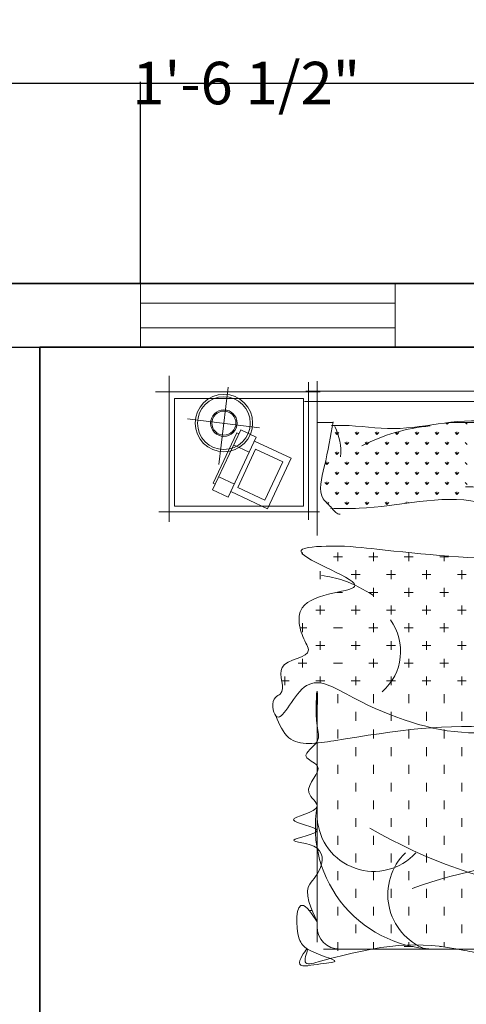
# Model space of a CAD drawing. Units: inches. Extents: x -26 to 575, y -18 to 513.
# Tile 26 of 28: x 376 to 439, y 374 to 513. Entities that reach past the tile are written whole.
import ezdxf

# ---------------------------------------------------------------- set-up
doc = ezdxf.new("R2010")
doc.units = ezdxf.units.IN
doc.header["$MEASUREMENT"] = 0
for name, color, linetype, lineweight in [('A-ANNO-DIMS', 2, 'Continuous', 18), ('A-GLAZ', 4, 'Continuous', 18), ('A-WALL', 7, 'Continuous', 35), ('Furniture', 8, 'Continuous', 15)]:
    doc.layers.add(name, color=color, linetype=linetype, lineweight=lineweight)
doc.styles.get("Standard").update_dxf_attribs({"font": 'arial.ttf', "height": 6})
doc.dimstyles.get("Standard").update_dxf_attribs({"dimtxt": 6, "dimasz": 0.18, "dimexe": 0.18, "dimexo": 0.0625, "dimgap": 0.09, "dimtad": 0, "dimtih": 1, "dimtoh": 1, "dimzin": 0, "dimdsep": 46, "dimlunit": 3, "dimtxsty": 'Standard', "dimcen": 0.09, "dimadec": 0, "dimazin": 0, "dimtfac": 1, "dimtofl": 0, "dimtmove": 0, "dimatfit": 3, "dimfxl": 1, "dimtolj": 1, "dimtzin": 0, "dimarcsym": 0})

# ---------------------------------------------------------------- blocks, each defined once
blk = doc.blocks.new('*D1')
at = {"layer": 'A-ANNO-DIMS', "color": 0, "lineweight": -2, "transparency": 16777216}
for p, q in [((18.18, 475.57), (18.18, 503.94)), ((18.36, 503.76), (264.87, 503.76)), ((522, 503.76), (275.48, 503.76)), ((522.18, 475.57), (522.18, 503.94))]:
    blk.add_line(p, q, dxfattribs=at)
at = {"layer": 'A-ANNO-DIMS', "color": 0, "transparency": 16777216}
for points in [[(18.36, 503.79), (18.36, 503.73), (18.18, 503.76)], [(522, 503.79), (522, 503.73), (522.18, 503.76)]]:
    blk.add_solid(points, dxfattribs=at)
at = {"layer": 'Defpoints', "color": 0, "transparency": 16777216}
for p in [(522.18, 503.76), (18.18, 475.51), (522.18, 475.51)]:
    blk.add_point(p, dxfattribs=at)
at = {"layer": 'A-ANNO-DIMS', "color": 0, "transparency": 16777216, "insert": (270.18, 503.76), "char_height": 6, "attachment_point": 5}
blk.add_mtext("\\A1;42'", dxfattribs=at)
blk = doc.blocks.new('BED-DOUBLE-WITH-NIGHTSTANDS')
for p, q in [((1.93, 83.36), (1.93, 62.76)), ((21.61, 63.03), (21.61, 82.46)), ((22.83, 60.83), (22.83, 82.62)), ((23.23, 81.08), (0, 81.08)), ((10.27, 81.76), (8.94, 70.83)), ((21.24, 81.17), (81.88, 81.17)), ((20.89, 80.15), (2.67, 80.15)), ((2.67, 80.15), (2.67, 64.97)), ((20.89, 64.97), (20.89, 80.15)), ((82.67, 79.72), (21.06, 79.72)), ((14.67, 76.01), (4.51, 77.26)), ((25.06, 76.76), (22.83, 76.76)), ((41.17, 76.51), (40.96, 76.72)), ((41.17, 76.51), (41.43, 76.77)), ((41.17, 76.51), (41.17, 76.74)), ((56.23, 76.76), (41.36, 76.76)), ((44, 76.51), (43.73, 76.77)), ((8.06, 67.24), (12.03, 75.72)), ((11.46, 75.32), (8.12, 68.2)), ((11.77, 75.18), (11.46, 75.32)), ((12.03, 75.72), (14.23, 74.69)), ((25.61, 75.09), (25.35, 75.36)), ((25.61, 75.09), (25.61, 75.47)), ((25.61, 75.09), (25.88, 75.36)), ((28.44, 75.09), (28.18, 75.36)), ((28.44, 75.09), (28.44, 75.47)), ((28.44, 75.09), (28.71, 75.36)), ((31.27, 75.09), (31, 75.36)), ((31.27, 75.09), (31.27, 75.47)), ((31.27, 75.09), (31.53, 75.36)), ((34.1, 75.09), (33.83, 75.36)), ((34.1, 75.09), (34.1, 75.47)), ((34.1, 75.09), (34.36, 75.36)), ((36.93, 75.09), (36.66, 75.36)), ((36.93, 75.09), (36.93, 75.47)), ((36.93, 75.09), (37.19, 75.36)), ((39.75, 75.09), (39.49, 75.36)), ((39.75, 75.09), (39.75, 75.47)), ((39.75, 75.09), (40.02, 75.36)), ((42.58, 75.09), (42.32, 75.36)), ((42.58, 75.09), (42.58, 75.47)), ((42.58, 75.09), (42.85, 75.36)), ((14.23, 74.69), (10.26, 66.21)), ((19.14, 71.73), (13.98, 74.14)), ((27.03, 73.68), (26.76, 73.94)), ((27.03, 73.68), (27.03, 74.05)), ((27.03, 73.68), (27.29, 73.94)), ((29.85, 73.68), (29.59, 73.94)), ((29.85, 73.68), (30.12, 73.94)), ((29.86, 73.68), (29.86, 74.05)), ((32.68, 73.68), (32.42, 73.94)), ((32.68, 73.68), (32.68, 74.05)), ((32.68, 73.68), (32.95, 73.94)), ((35.51, 73.68), (35.25, 73.94)), ((35.51, 73.68), (35.51, 74.05)), ((35.51, 73.68), (35.78, 73.94)), ((38.34, 73.68), (38.07, 73.94)), ((38.34, 73.68), (38.34, 74.05)), ((38.34, 73.68), (38.61, 73.94)), ((41.17, 73.68), (40.9, 73.94)), ((41.17, 73.68), (41.17, 74.05)), ((41.17, 73.68), (41.43, 73.94)), ((44, 73.68), (43.73, 73.94)), ((13.24, 72.57), (11.03, 73.6)), ((14.13, 73), (11.6, 67.59)), ((17.98, 71.2), (14.13, 73)), ((25.61, 72.26), (25.35, 72.53)), ((25.61, 72.26), (25.61, 72.64)), ((25.61, 72.26), (25.88, 72.53)), ((28.44, 72.26), (28.18, 72.53)), ((28.44, 72.26), (28.44, 72.64)), ((28.44, 72.26), (28.71, 72.53)), ((31.27, 72.26), (31, 72.53)), ((31.27, 72.26), (31.27, 72.64)), ((31.27, 72.26), (31.53, 72.53)), ((34.1, 72.26), (33.83, 72.53)), ((34.1, 72.26), (34.1, 72.64)), ((34.1, 72.26), (34.36, 72.53)), ((36.93, 72.26), (36.66, 72.53)), ((36.93, 72.26), (36.93, 72.64)), ((36.93, 72.26), (37.19, 72.53)), ((39.75, 72.26), (39.49, 72.53)), ((39.75, 72.26), (39.75, 72.64)), ((39.75, 72.26), (40.02, 72.53)), ((42.58, 72.26), (42.32, 72.53)), ((42.58, 72.26), (42.58, 72.64)), ((42.58, 72.26), (42.85, 72.53)), ((15.45, 65.79), (17.98, 71.2)), ((15.8, 64.6), (19.14, 71.73)), ((24.2, 70.85), (23.97, 71.08)), ((24.2, 70.85), (24.2, 71.23)), ((24.2, 70.85), (24.46, 71.12)), ((27.03, 70.85), (26.76, 71.12)), ((27.03, 70.85), (27.03, 71.23)), ((27.03, 70.85), (27.29, 71.12)), ((29.85, 70.85), (29.59, 71.12)), ((29.85, 70.85), (30.12, 71.12)), ((29.86, 70.85), (29.86, 71.23)), ((32.68, 70.85), (32.42, 71.12)), ((32.68, 70.85), (32.68, 71.23)), ((32.68, 70.85), (32.95, 71.12)), ((35.51, 70.85), (35.25, 71.12)), ((35.51, 70.85), (35.51, 71.23)), ((35.51, 70.85), (35.78, 71.12)), ((38.34, 70.85), (38.07, 71.12)), ((38.34, 70.85), (38.34, 71.23)), ((38.34, 70.85), (38.61, 71.12)), ((41.17, 70.85), (40.9, 71.12)), ((41.17, 70.85), (41.17, 71.23)), ((41.17, 70.85), (41.43, 71.12)), ((44, 70.85), (43.73, 71.12)), ((25.61, 69.44), (25.35, 69.7)), ((25.61, 69.44), (25.61, 69.81)), ((25.61, 69.44), (25.88, 69.7)), ((28.44, 69.44), (28.18, 69.7)), ((28.44, 69.44), (28.44, 69.81)), ((28.44, 69.44), (28.71, 69.7)), ((31.27, 69.44), (31, 69.7)), ((31.27, 69.44), (31.27, 69.81)), ((31.27, 69.44), (31.53, 69.7)), ((34.1, 69.44), (33.83, 69.7)), ((34.1, 69.44), (34.1, 69.81)), ((34.1, 69.44), (34.36, 69.7)), ((36.93, 69.44), (36.66, 69.7)), ((36.93, 69.44), (36.93, 69.81)), ((36.93, 69.44), (37.19, 69.7)), ((39.75, 69.44), (39.49, 69.7)), ((39.75, 69.44), (39.75, 69.81)), ((39.75, 69.44), (40.02, 69.7)), ((42.58, 69.44), (42.32, 69.7)), ((42.58, 69.44), (42.58, 69.81)), ((42.58, 69.44), (42.85, 69.7)), ((8.12, 68.2), (8.43, 68.05)), ((11.14, 68.07), (8.93, 69.1)), ((24.2, 68.02), (23.93, 68.29)), ((24.2, 68.02), (24.2, 68.4)), ((24.2, 68.02), (24.46, 68.29)), ((27.03, 68.02), (26.76, 68.29)), ((27.03, 68.02), (27.03, 68.4)), ((27.03, 68.02), (27.29, 68.29)), ((29.85, 68.02), (29.59, 68.29)), ((29.85, 68.02), (30.12, 68.29)), ((29.86, 68.02), (29.86, 68.4)), ((32.68, 68.02), (32.42, 68.29)), ((32.68, 68.02), (32.68, 68.4)), ((32.68, 68.02), (32.95, 68.29)), ((35.51, 68.02), (35.25, 68.29)), ((35.51, 68.02), (35.51, 68.4)), ((35.51, 68.02), (35.78, 68.29)), ((38.34, 68.02), (38.07, 68.29)), ((38.34, 68.02), (38.34, 68.4)), ((38.34, 68.02), (38.61, 68.29)), ((41.17, 68.02), (40.9, 68.29)), ((41.17, 68.02), (41.17, 68.4)), ((41.17, 68.02), (41.43, 68.29)), ((44, 68.02), (43.73, 68.29)), ((10.26, 66.21), (8.06, 67.24)), ((10.64, 67.02), (15.8, 64.6)), ((11.6, 67.59), (15.45, 65.79)), ((25.61, 66.61), (25.35, 66.87)), ((25.61, 66.61), (25.61, 66.98)), ((25.61, 66.61), (25.88, 66.87)), ((28.44, 66.61), (28.18, 66.87)), ((28.44, 66.61), (28.44, 66.98)), ((28.44, 66.61), (28.71, 66.87)), ((31.27, 66.61), (31, 66.87)), ((31.27, 66.61), (31.27, 66.98)), ((31.27, 66.61), (31.53, 66.87)), ((34.1, 66.61), (33.83, 66.87)), ((34.1, 66.61), (34.1, 66.98)), ((34.1, 66.61), (34.36, 66.87)), ((36.93, 66.61), (36.66, 66.87)), ((36.93, 66.61), (36.93, 66.98)), ((36.93, 66.61), (37.19, 66.87)), ((39.75, 66.61), (39.49, 66.87)), ((39.75, 66.61), (39.75, 66.98)), ((39.75, 66.61), (40.02, 66.87)), ((42.58, 66.61), (42.32, 66.87)), ((42.58, 66.61), (42.58, 66.98)), ((42.58, 66.61), (42.85, 66.87)), ((24.2, 65.39), (24.2, 65.57)), ((24.29, 65.29), (24.46, 65.46)), ((27.03, 65.19), (26.76, 65.46)), ((27.03, 65.19), (27.03, 65.57)), ((27.03, 65.19), (27.29, 65.46)), ((29.85, 65.19), (29.59, 65.46)), ((29.85, 65.19), (30.12, 65.46)), ((29.86, 65.19), (29.86, 65.57)), ((32.68, 65.19), (32.42, 65.46)), ((32.68, 65.19), (32.68, 65.57)), ((32.68, 65.19), (32.95, 65.46)), ((35.33, 65.37), (35.25, 65.46)), ((35.51, 65.39), (35.51, 65.57)), ((35.74, 65.42), (35.78, 65.46)), ((0.45, 64.15), (23.14, 64.15)), ((2.67, 64.97), (20.89, 64.97)), ((20.77, 58.21), (20.77, 58.42)), ((25.77, 57.17), (25.77, 58.42)), ((30.77, 57.17), (30.77, 58.42)), ((35.77, 57.17), (35.77, 58.41)), ((21.39, 57.79), (21.31, 57.79)), ((26.39, 57.79), (25.14, 57.79)), ((31.39, 57.79), (30.14, 57.79)), ((36.39, 57.79), (35.14, 57.79)), ((41.39, 57.79), (40.14, 57.79)), ((40.77, 57.17), (40.77, 57.97)), ((23.27, 54.64), (23.27, 55.76)), ((28.27, 54.67), (28.27, 55.92)), ((33.27, 54.67), (33.27, 55.92)), ((38.27, 54.67), (38.27, 55.92)), ((43.27, 54.67), (43.27, 55.92)), ((28.89, 55.29), (27.64, 55.29)), ((33.89, 55.29), (32.64, 55.29)), ((38.89, 55.29), (37.64, 55.29)), ((43.89, 55.29), (42.64, 55.29)), ((30.77, 52.17), (30.77, 53.42)), ((35.77, 52.17), (35.77, 53.42)), ((40.77, 52.17), (40.77, 53.42)), ((26.39, 52.79), (25.62, 52.79)), ((31.39, 52.79), (30.14, 52.79)), ((36.39, 52.79), (35.14, 52.79)), ((41.39, 52.79), (40.14, 52.79)), ((23.89, 50.29), (22.64, 50.29)), ((23.27, 49.67), (23.27, 50.92)), ((28.89, 50.29), (27.64, 50.29)), ((28.27, 49.67), (28.27, 50.92)), ((33.89, 50.29), (32.64, 50.29)), ((33.27, 49.67), (33.27, 50.92)), ((38.89, 50.29), (37.64, 50.29)), ((38.27, 49.67), (38.27, 50.92)), ((43.89, 50.29), (42.64, 50.29)), ((43.27, 49.67), (43.27, 50.92)), ((21.39, 47.79), (20.41, 47.79)), ((20.77, 47.17), (20.77, 48.42)), ((26.39, 47.79), (25.14, 47.79)), ((31.39, 47.79), (30.14, 47.79)), ((30.77, 47.17), (30.77, 48.42)), ((36.39, 47.79), (35.14, 47.79)), ((35.77, 47.17), (35.77, 48.42)), ((41.39, 47.79), (40.14, 47.79)), ((40.77, 47.17), (40.77, 48.42)), ((23.27, 44.67), (23.27, 45.92)), ((28.27, 44.67), (28.27, 45.92)), ((33.27, 44.67), (33.27, 45.92)), ((38.27, 44.67), (38.27, 45.92)), ((43.27, 44.67), (43.27, 45.92)), ((23.89, 45.29), (22.64, 45.29)), ((28.89, 45.29), (27.64, 45.29)), ((33.89, 45.29), (32.64, 45.29)), ((38.89, 45.29), (37.64, 45.29)), ((43.89, 45.29), (42.64, 45.29)), ((20.77, 42.17), (20.77, 43.42)), ((30.77, 42.17), (30.77, 43.42)), ((35.77, 42.17), (35.77, 43.42)), ((40.77, 42.17), (40.77, 43.42)), ((21.39, 42.79), (20.14, 42.79)), ((26.39, 42.79), (25.14, 42.79)), ((31.39, 42.79), (30.14, 42.79)), ((36.39, 42.79), (35.14, 42.79)), ((41.39, 42.79), (40.14, 42.79)), ((18.27, 39.67), (18.27, 40.92)), ((23.27, 39.99), (23.27, 40.92)), ((28.27, 39.67), (28.27, 40.92)), ((33.27, 39.67), (33.27, 40.92)), ((38.27, 39.67), (38.27, 40.92)), ((43.27, 39.67), (43.27, 40.92)), ((18.89, 40.29), (17.83, 40.29)), ((23.89, 40.29), (22.64, 40.29)), ((28.89, 40.29), (27.64, 40.29)), ((33.89, 40.29), (32.64, 40.29)), ((38.89, 40.29), (37.64, 40.29)), ((43.89, 40.29), (42.64, 40.29)), ((22.83, 3.42), (22.83, 38.86)), ((25.77, 37.17), (25.77, 38.42)), ((30.77, 37.17), (30.77, 38.42)), ((35.77, 37.17), (35.77, 38.42)), ((40.77, 37.17), (40.77, 38.42)), ((17.66, 35.29), (17.64, 35.29)), ((28.27, 34.67), (28.27, 35.92)), ((33.27, 34.67), (33.27, 35.92)), ((38.27, 34.67), (38.27, 35.92)), ((43.27, 34.67), (43.27, 35.92)), ((25.77, 32.17), (25.77, 33.42)), ((30.77, 32.17), (30.77, 33.42)), ((35.77, 32.17), (35.77, 33.42)), ((40.77, 32.17), (40.77, 33.42)), ((28.27, 29.67), (28.27, 30.92)), ((33.27, 29.67), (33.27, 30.92)), ((38.27, 29.67), (38.27, 30.92)), ((43.27, 29.67), (43.27, 30.92)), ((25.77, 27.17), (25.77, 28.42)), ((30.77, 27.17), (30.77, 28.42)), ((35.77, 27.17), (35.77, 28.42)), ((40.77, 27.17), (40.77, 28.42)), ((28.27, 24.67), (28.27, 25.92)), ((33.27, 24.67), (33.27, 25.92)), ((38.27, 24.67), (38.27, 25.92)), ((43.27, 24.67), (43.27, 25.92)), ((25.77, 22.17), (25.77, 23.42)), ((30.77, 22.17), (30.77, 23.42)), ((35.77, 22.17), (35.77, 23.42)), ((40.77, 22.17), (40.77, 23.42)), ((28.27, 19.67), (28.27, 20.92)), ((33.27, 19.67), (33.27, 20.92)), ((38.27, 19.67), (38.27, 20.92)), ((43.27, 19.67), (43.27, 20.92)), ((25.77, 17.17), (25.77, 18.42)), ((30.77, 17.17), (30.77, 18.42)), ((35.77, 17.17), (35.77, 18.42)), ((40.77, 17.17), (40.77, 18.42)), ((28.27, 14.67), (28.27, 15.92)), ((33.27, 14.67), (33.27, 15.92)), ((38.27, 14.67), (38.27, 15.92)), ((43.27, 14.67), (43.27, 15.92)), ((25.77, 12.17), (25.77, 13.42)), ((30.77, 12.17), (30.77, 13.42)), ((35.77, 12.17), (35.77, 13.42)), ((40.77, 12.17), (40.77, 13.42)), ((28.27, 9.67), (28.27, 10.92)), ((33.27, 9.67), (33.27, 10.92)), ((38.27, 9.67), (38.27, 10.92)), ((43.27, 9.67), (43.27, 10.92)), ((25.77, 7.17), (25.77, 8.42)), ((30.77, 7.17), (30.77, 8.42)), ((35.77, 7.17), (35.77, 8.42)), ((40.77, 7.17), (40.77, 8.42)), ((22.12, 7.87), (21.71, 7.87)), ((28.27, 4.67), (28.27, 5.92)), ((33.27, 4.67), (33.27, 5.92)), ((38.27, 4.67), (38.27, 5.92)), ((43.27, 4.67), (43.27, 5.92)), ((25.77, 2.17), (25.77, 3.42)), ((30.77, 2.46), (30.77, 3.42)), ((36.39, 2.79), (35.14, 2.79)), ((35.77, 3), (35.77, 3.42)), ((40.4, 2.79), (40.14, 2.79)), ((40.77, 2.75), (40.77, 3.42)), ((85.58, 2.43), (23.7, 2.43))]:
    blk.add_line(p, q)
for radius in [4.06, 3.73, 1.87, 1.7]:
    blk.add_circle((9.65, 76.68), radius)
for centre, radius, start, end in [((18.64, 72.67), 7.53, 354.3248, 27.7728), ((41.09, 50.38), 26, 95.0264, 117.3299), ((44.42, 57.1), 10.59, 48.8713, 93.3448), ((27.06, 44.47), 7.56, 311.0401, 36.1384), ((39.78, 19.64), 17.21, 170.0678, 270.9321), ((30.83, 21.41), 8.01, 183.5361, 317.8486), ((66.97, 82.6), 72.97, 239.8126, 282.5472), ((41.05, 10.13), 8.24, 134.2353, 249.0585), ((61.48, -60.53), 75.85, 75.7143, 109.4459), ((25.97, 5.58), 3.15, 180, 270)]:
    blk.add_arc(centre, radius, start, end)
for points, knots in [([(25.07, 76.86), (24.73, 74.84), (24.15, 71.41), (22.76, 66.41), (24.85, 64.9), (25.6, 63.75), (26.07, 63.83)], [0, 0, 0, 0, 6.47304, 11.006869, 12.799679, 14.2185, 14.2185, 14.2185, 14.2185]), ([(24.71, 64.66), (26.06, 64.63), (33, 64.48), (41.95, 67.2), (49.02, 64.48), (52.79, 64.86), (50.63, 69.88), (50.43, 72.76), (51.76, 76.03), (43.45, 78.05), (36.59, 75.07), (28.31, 76.39), (25.37, 76.36), (24.84, 76.35)], [0, 0, 0, 0, 4.049674, 20.880819, 25.932041, 26.821979, 31.217024, 36.043065, 37.533831, 40.150607, 55.448466, 62.672935, 64.278467, 64.278467, 64.278467, 64.278467]), ([(83.91, 58.07), (84.56, 56.74), (85.58, 54.64), (82.28, 53.65), (82.99, 50.72), (85.33, 50.53), (84.9, 48.23), (82.06, 47.25), (85.77, 45.87), (88.76, 44.17), (85.37, 42.03), (87.05, 39.3), (78.86, 37.34), (72.98, 51.01), (54.08, 29.24), (35.91, 32.92), (20.82, 41.99), (17.17, 32.57), (16.24, 37.8), (18.71, 38.79), (15.91, 43.44), (22.37, 43.45), (20.93, 46.18), (20.19, 47.95), (20.32, 52.93), (35.13, 52.6), (16.25, 58.94), (26.31, 59.48), (35.16, 58.38), (54.32, 56.67), (69.44, 58.46), (82.07, 60.88), (83.53, 58.65), (83.91, 58.07)], [0, 0, 0, 0, 3.481099, 5.475811, 8.043407, 9.436812, 11.330727, 12.888379, 16.258255, 18.252967, 21.734596, 23.018392, 26.087149, 38.445812, 54.5649, 86.600283, 92.594507, 98.286547, 100.905288, 101.70342, 105.471876, 109.954916, 110.954151, 113.598333, 116.114301, 124.231953, 133.25029, 137.509046, 143.991555, 164.906349, 189.961005, 195.579007, 197.573325, 197.573325, 197.573325, 197.573325]), ([(23.43, 55.19), (24.49, 55), (27.11, 54.54), (29.42, 53.18), (30.79, 52.36)], [0, 0, 0, 0, 3.194191, 7.94245, 7.94245, 7.94245, 7.94245]), ([(82.95, 38.85), (82.91, 38.17), (82.85, 36.97), (81.76, 35.43), (82.66, 33.92), (82.17, 32.16), (83.17, 30.81), (83.54, 28.6), (81.84, 26.13), (84.59, 22.62), (82.27, 21.86), (82.5, 20.48), (82.77, 18.98), (83.36, 17.21), (83.5, 15.41), (82.61, 14.09), (82.87, 12.46), (82.71, 11.04), (83.72, 9.61), (82.91, 7.55), (83.23, 5.58), (83.08, 3.39), (85.08, 3.34), (83.88, 2.36), (83.09, 3.04), (82.19, 1.93), (80.71, 0.69), (78.27, 1.05), (76.16, 2.63), (73.68, 2.58), (71.48, 0.95), (69.05, 1.47), (65.15, 1.19), (60.81, 2), (56.05, 2.59), (52.45, 0.27), (49.19, 1.51), (46.12, 1.7), (37.69, 3.67), (31.84, 3.18), (20.44, -0.09), (22.21, 3.75), (19.18, -0.44), (22.91, 0.39), (27.14, 0.63), (21.63, 1.85), (19.68, 4.27), (19.87, 11.16), (24.26, 3.84), (20.3, 10.76), (23.26, 12.85), (24.33, 17.43), (16.78, 17.59), (25.96, 19.23), (16.2, 20.68), (24.67, 22.01), (20.04, 24.96), (24.6, 28.15), (20.03, 29.6), (23.48, 31.6), (22.43, 34.55), (22.92, 41.18), (22.85, 37.06), (22.83, 35.35)], [0, 0, 0, 0, 2.033881, 3.581387, 5.07489, 6.704853, 8.655612, 9.757262, 13.24098, 16.903694, 18.063816, 18.788243, 20.635227, 22.875483, 24.324336, 25.871843, 27.320698, 29.140811, 29.950855, 32.312207, 34.847704, 36.565952, 37.541804, 38.447727, 39.194923, 40.100844, 41.912688, 45.194843, 46.251388, 49.875946, 51.496686, 54.215105, 56.7523, 63.316606, 67.484853, 70.581422, 75.324573, 76.965649, 79.915763, 100.671038, 102.483321, 104.317501, 106.523635, 109.038061, 111.571263, 115.809372, 117.667229, 122.411431, 125.445794, 129.976907, 132.758854, 136.424739, 139.918708, 143.481583, 147.135325, 151.002466, 153.252794, 157.23352, 159.244583, 161.905351, 164.097269, 169.015093, 172.531686, 172.531686, 172.531686, 172.531686]), ([(82.45, 38.63), (79.86, 38.49), (74.81, 38.21), (68.7, 28.86), (57.63, 32.1), (43.09, 34.7), (32.13, 32.98), (18.89, 30.82), (17.48, 34.15), (16.98, 35.35)], [0, 0, 0, 0, 7.385187, 14.402621, 29.694422, 35.583277, 59.348121, 65.733553, 69.320983, 69.320983, 69.320983, 69.320983])]:
    blk.add_open_spline(points, degree=3, knots=knots)
blk = doc.blocks.new('WINDOW-36IN')
for p, q in [((36, 9), (0, 9)), ((0, 9), (0, 0)), ((36, 0), (36, 9)), ((36, 6.25), (0, 6.25)), ((36, 0), (36, 4.5)), ((36, 2.75), (0, 2.75)), ((0, 0), (36, 0))]:
    blk.add_line(p, q)
blk = doc.blocks.new('*D12')
at = {"layer": 'A-ANNO-DIMS', "color": 0, "lineweight": -2, "transparency": 16777216}
for p, q in [((143.38, 375.47), (143.38, 359.76)), ((247.35, 375.47), (247.35, 359.76)), ((143.56, 359.94), (247.17, 359.94)), ((247.35, 359.94), (247.53, 359.94))]:
    blk.add_line(p, q, dxfattribs=at)
at = {"layer": 'A-ANNO-DIMS', "color": 0, "transparency": 16777216}
for points in [[(143.56, 359.97), (143.56, 359.91), (143.38, 359.94)], [(247.17, 359.97), (247.17, 359.91), (247.35, 359.94)]]:
    blk.add_solid(points, dxfattribs=at)
at = {"layer": 'Defpoints', "color": 0, "transparency": 16777216}
for p in [(143.38, 375.53), (247.35, 375.53), (247.35, 359.94)]:
    blk.add_point(p, dxfattribs=at)
at = {"layer": 'A-ANNO-DIMS', "color": 0, "transparency": 16777216, "insert": (329.1, 359.94), "char_height": 6, "attachment_point": 5}
blk.add_mtext('\\A1;DOUBLE BED & NIGHTSTANDS 8\'-8" TYP.', dxfattribs=at)
blk = doc.blocks.new('*D32')
at = {"layer": 'A-ANNO-DIMS', "color": 0, "lineweight": -2, "transparency": 16777216}
for p, q in [((374.18, 466.57), (374.18, 503.99)), ((374.36, 503.81), (392.7, 503.81)), ((392.88, 475.57), (392.88, 503.99)), ((392.88, 503.81), (393.06, 503.81))]:
    blk.add_line(p, q, dxfattribs=at)
at = {"layer": 'A-ANNO-DIMS', "color": 0, "transparency": 16777216}
for points in [[(374.36, 503.84), (374.36, 503.78), (374.18, 503.81)], [(392.7, 503.84), (392.7, 503.78), (392.88, 503.81)]]:
    blk.add_solid(points, dxfattribs=at)
at = {"layer": 'Defpoints', "color": 0, "transparency": 16777216}
for p in [(392.88, 503.81), (392.88, 475.51), (374.18, 466.51)]:
    blk.add_point(p, dxfattribs=at)
at = {"layer": 'A-ANNO-DIMS', "color": 0, "transparency": 16777216, "insert": (407.83, 503.81), "char_height": 6, "attachment_point": 5}
blk.add_mtext('\\A1;1\'-6 1/2"', dxfattribs=at)
blk = doc.blocks.new('*D49')
at = {"layer": 'A-ANNO-DIMS', "color": 0, "lineweight": -2, "transparency": 16777216}
for p, q in [((278.24, 466.51), (550.66, 466.51)), ((550.48, 466.33), (550.48, 403.66)), ((550.48, 334.69), (550.48, 397.35)), ((278.24, 334.51), (550.66, 334.51))]:
    blk.add_line(p, q, dxfattribs=at)
at = {"layer": 'A-ANNO-DIMS', "color": 0, "transparency": 16777216}
for points in [[(550.45, 466.33), (550.51, 466.33), (550.48, 466.51)], [(550.45, 334.69), (550.51, 334.69), (550.48, 334.51)]]:
    blk.add_solid(points, dxfattribs=at)
at = {"layer": 'Defpoints', "color": 0, "transparency": 16777216}
for p in [(278.18, 466.51), (550.48, 466.51), (278.18, 334.51)]:
    blk.add_point(p, dxfattribs=at)
at = {"layer": 'A-ANNO-DIMS', "color": 0, "transparency": 16777216, "insert": (550.48, 400.51), "char_height": 6, "attachment_point": 5}
blk.add_mtext('\\A1;11\'-0"', dxfattribs=at)

msp = doc.modelspace()

# ---------------------------------------------------------------- linework, layer by layer
at = {"layer": 'A-WALL'}
for p in [(513.177, 466.508), (378.677, 334.508)]:
    msp.add_line(p, (378.677, 466.508), dxfattribs=at)
msp.add_lwpolyline([(18.177, 19.508), (522.177, 19.508), (522.177, 475.508), (18.177, 475.508)], close=True, dxfattribs=at)

# ---------------------------------------------------------------- block references
at = {"layer": 'A-GLAZ'}
msp.add_blockref('WINDOW-36IN', (392.879, 466.508), dxfattribs=at)
at = {"layer": 'Furniture'}
msp.add_blockref('BED-DOUBLE-WITH-NIGHTSTANDS', (395.028, 379.13), dxfattribs=at)

# ---------------------------------------------------------------- dimensions: what is measured, and where the dimension line sits
at = {"layer": 'A-ANNO-DIMS'}
for base, p1, p2, override, picture, middle in [((392.879, 503.808), (374.177, 466.508), (392.879, 475.508), {"dimdec": 1, "dimlfac": 1, "dimrnd": 0, "dimzin": 1, "dimdsep": 46, "dimlunit": 4, "dimfrac": 2}, '*D32', (407.832, 503.808)), ((522.177, 503.757), (18.177, 475.508), (522.177, 475.508), {"dimclrd": 0, "dimclre": 0, "dimclrt": 0}, '*D1', (270.177, 503.757))]:
    dim = msp.add_linear_dim(base=base, p1=p1, p2=p2, dimstyle='Standard', override=override, dxfattribs=at)
    dim.commit()
    dim.dimension.update_dxf_attribs({"geometry": picture, "text_midpoint": middle})
dim = msp.add_linear_dim(base=(550.477, 466.508), p1=(278.177, 334.508), p2=(278.177, 466.508), angle=90, dimstyle='Standard', override={"dimdec": 1, "dimlfac": 1, "dimrnd": 0, "dimzin": 1, "dimdsep": 46, "dimlunit": 4, "dimfrac": 2}, dxfattribs=at)
dim.commit()
dim.dimension.update_dxf_attribs({"geometry": '*D49', "text_midpoint": (550.477, 400.508)})
dim = msp.add_linear_dim(base=(247.348, 359.935), p1=(143.378, 375.531), p2=(247.348, 375.531), text='DOUBLE BED & NIGHTSTANDS <> TYP.', dimstyle='Standard', override={"dimdec": 1, "dimlfac": 1, "dimrnd": 0, "dimzin": 1, "dimdsep": 46, "dimlunit": 4, "dimfrac": 2}, dxfattribs=at)
dim.commit()
dim.dimension.update_dxf_attribs({"geometry": '*D12', "text_midpoint": (329.097, 359.935)})

doc.saveas('drawing.dxf')
